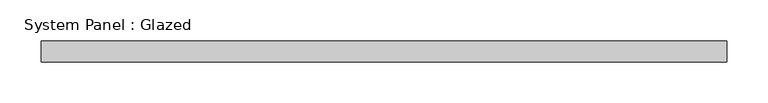
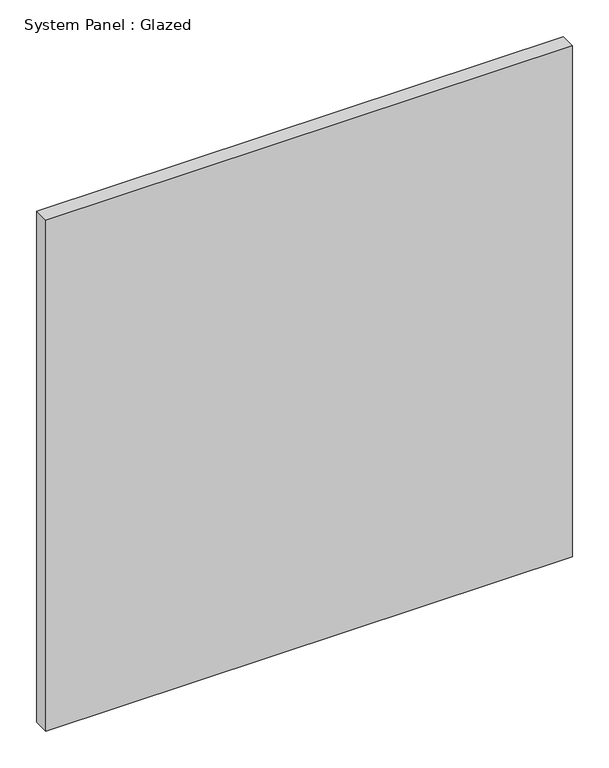
"""IFC4 building model written with IfcOpenShell, lengths in millimetres: plate geometry, System Panel : Glazed."""

from ifc_helpers import new_model, si_unit, origin, origin_with_axes, place, context, project, spatial, polyline, outline, extrude, source, transform, mapped, element, save


def system_panel_glazed_1cb891c7(model_context):
    return source(origin(), model_context, "Body", "SweptSolid", [
        extrude(outline(polyline([(415.925, 19.05), (-415.925, 19.05), (-415.925, 44.45), (415.925, 44.45), (415.925, 19.05)])), origin_with_axes(), (0.0, 0.0, 1.0), 853.0145651),
    ])


if __name__ == "__main__":
    model = new_model("IFC4")
    model_context = context("Model", 3, world=origin())
    ifc_project = project(units=[si_unit("LENGTHUNIT", "METRE", prefix="MILLI")], contexts=[model_context])
    site = spatial("IfcSite", under=ifc_project)
    building = spatial("IfcBuilding", under=site)
    placement = place(None, origin())
    system_panel_glazed_shape = system_panel_glazed_1cb891c7(model_context)
    element("IfcPlate", 1, ObjectType="System Panel : Glazed", at=placement, inside=building, context=model_context, shape_type="MappedRepresentation", body=[
        mapped(system_panel_glazed_shape, transform((0.0, 0.0, 0.0), x_axis=(1.0, 0.0, 0.0), y_axis=(0.0, 1.0, 0.0), z_axis=(0.0, 0.0, 1.0))),
    ])
    save(model, "model.ifc")

# Revit data of these elements
# Type "System Panel : Glazed"
#   Construction Type Id = "GSP4R"
#   Analytic Construction = "1/8 in Pilkington single glazing"
#   Visual Light Transmittance = 0.9
#   Solar Heat Gain Coefficient = 0.86
#   Heat Transfer Coefficient (U) = 1.18115 BTU/(h·ft²·°F)
#   Define Thermal Properties by = 1
# Element 1 (IfcPlate, "System Panel : Glazed")
#   Materials on its faces: "Glass"
# Materials
#   "Glass": class "Glass", colour RGB 0 128 192, transparency 0.75, Description = "Soda Lime Glass", Cost = 0
